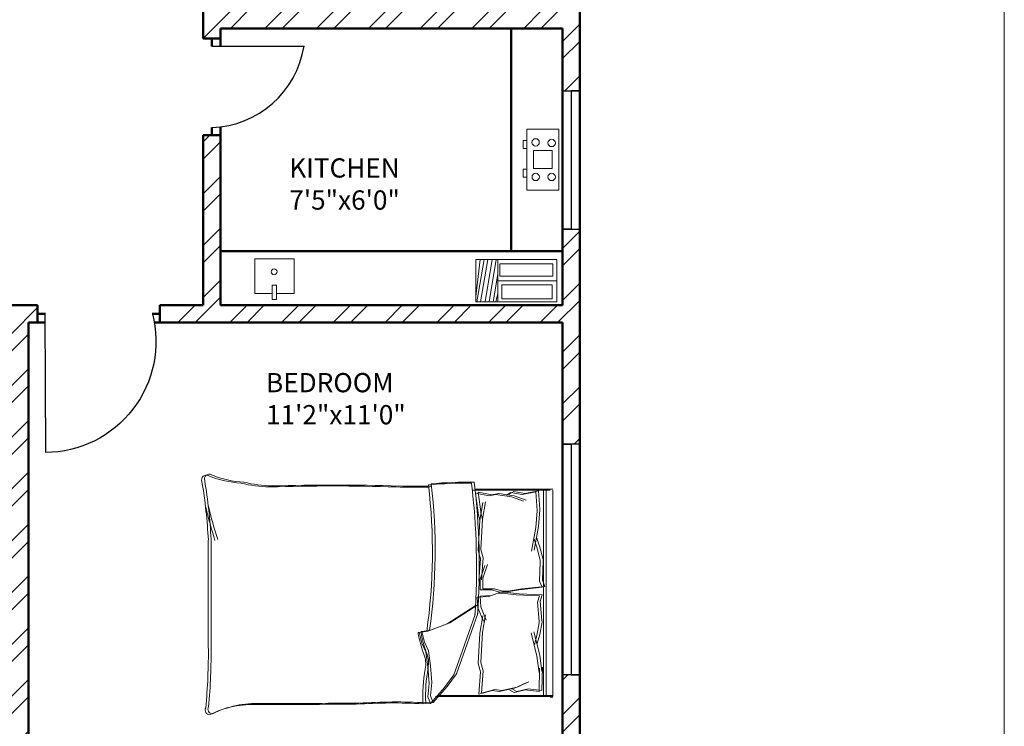
# Model space of a CAD drawing. Units: inches. Extents: x 1901 to 2863, y 888 to 2433.
# Tile 34 of 91: x 2607 to 2863, y 1291 to 1474. Entities that reach past the tile are written whole.
import ezdxf

# ---------------------------------------------------------------- set-up
doc = ezdxf.new("R2010")
doc.units = ezdxf.units.IN
for name, color, linetype, lineweight in [('A-AREA-IDEN', 7, 'Continuous', 18), ('A-DOOR', 4, 'Continuous', 25), ('A-FLOR-FIXT', 9, 'Continuous', 18), ('A-FURN', 8, 'Continuous', 18), ('A-GLAZ', 3, 'Continuous', 25), ('A-WALL', 7, 'Continuous', 50), ('A-WALL-PATT', 8, 'Continuous', 13)]:
    doc.layers.add(name, color=color, linetype=linetype, lineweight=lineweight)
doc.styles.get("Standard").update_dxf_attribs({"font": 'arial.ttf'})

# ---------------------------------------------------------------- blocks, each defined once
blk = doc.blocks.new('BED-DOUBLE')
for p, q in [((31.18, 59.32), (27.53, 55.16)), ((31.18, 59.32), (27.53, 55.16)), ((31.9, 59.58), (28.25, 55.42)), ((31.9, 59.58), (28.25, 55.42)), ((33.14, 59.41), (31.18, 59.32, 4.35)), ((33.14, 59.41), (31.18, 59.32, 4.35)), ((31.87, 57.59), (31.18, 59.32)), ((31.87, 57.59), (31.18, 59.32)), ((33.85, 59.67), (31.9, 59.58, 4.35)), ((33.85, 59.67), (31.9, 59.58, 4.35)), ((32.59, 57.85), (31.9, 59.58)), ((32.59, 57.85), (31.9, 59.58)), ((0.03, 57.78), (0.03, 4.12)), ((0.74, 57.78), (30.62, 57.78)), ((0.74, 57.78), (30.62, 57.78)), ((3.61, 56.48), (3.51, 50.42)), ((3.61, 56.48), (3.51, 50.42)), ((3.61, 56.48), (7.22, 56.06)), ((3.61, 56.48), (7.22, 56.06)), ((6.5, 55.8), (9.39, 56.47)), ((6.5, 55.8), (9.39, 56.47)), ((7.22, 56.06), (10.11, 56.73)), ((7.22, 56.06), (10.11, 56.73)), ((9.39, 56.47), (10.56, 55.89)), ((9.39, 56.47), (10.56, 55.89)), ((14.02, 56.48), (10.01, 55.58)), ((14.02, 56.48), (10.01, 55.58)), ((10.11, 56.73), (11.28, 56.15)), ((10.11, 56.73), (11.28, 56.15)), ((15.83, 56.27), (14.02, 56.48)), ((15.83, 56.27), (14.02, 56.48)), ((18.63, 56.89), (15.11, 56.01)), ((18.63, 56.88), (15.11, 56.01)), ((19.35, 57.14), (15.83, 56.27)), ((19.35, 57.14), (15.83, 56.27)), ((18.18, 51.12), (18.63, 56.89)), ((18.18, 51.12), (18.63, 56.88)), ((18.9, 51.38), (19.35, 57.14)), ((18.9, 51.38), (19.35, 57.14)), ((31.53, 54.12), (31.87, 57.59)), ((31.53, 54.12), (31.87, 57.59)), ((32.24, 54.37), (32.59, 57.85)), ((32.24, 54.37), (32.59, 57.85)), ((2.9, 56.23), (2.79, 50.16)), ((2.9, 56.23), (2.79, 50.16)), ((2.9, 56.23), (6.5, 55.8)), ((2.9, 56.23), (6.5, 55.8)), ((9.3, 55.33), (6.29, 54)), ((9.3, 55.33), (6.29, 54)), ((10.01, 55.58), (7.01, 54.26)), ((10.01, 55.58), (7.01, 54.26)), ((13.31, 56.23), (9.3, 55.33)), ((13.31, 56.23), (9.3, 55.33)), ((15.11, 56.01), (13.31, 56.23)), ((15.11, 56.01), (13.31, 56.23)), ((27.53, 55.16), (25.1, 51.86)), ((27.53, 55.16), (25.1, 51.86)), ((28.25, 55.42), (25.81, 52.11)), ((28.25, 55.42), (25.81, 52.11)), ((31.87, 49.77), (31.53, 54.12)), ((31.87, 49.77), (31.53, 54.12)), ((32.59, 50.03), (32.24, 54.37)), ((32.59, 50.03), (32.24, 54.37)), ((2.79, 50.16), (2.88, 51.29)), ((2.79, 50.16), (2.88, 51.29)), ((2.88, 51.29), (3.47, 47.02)), ((2.88, 51.29), (3.47, 47.02)), ((3.51, 50.42), (3.6, 51.54)), ((3.51, 50.42), (3.6, 51.54)), ((3.6, 51.54), (4.19, 47.28)), ((3.6, 51.54), (4.19, 47.28)), ((19.52, 49.18), (18.9, 51.38)), ((19.52, 49.18), (18.9, 51.38)), ((25.1, 51.86), (22.84, 45.6)), ((25.1, 51.86), (22.84, 45.6)), ((25.81, 52.11), (23.55, 45.85)), ((25.81, 52.11), (23.55, 45.85)), ((18.81, 48.92), (18.18, 51.12)), ((18.81, 48.92), (18.18, 51.12)), ((18.32, 41.05), (18.81, 48.92)), ((18.32, 41.05), (18.81, 48.92)), ((19.04, 41.31), (19.52, 49.18)), ((19.04, 41.31), (19.52, 49.18)), ((32.39, 45.94), (31.87, 49.77)), ((32.39, 45.94), (31.87, 49.77)), ((33.11, 46.2), (32.59, 50.03)), ((33.11, 46.2), (32.59, 50.03)), ((3.47, 47.02), (4.99, 40.94)), ((3.47, 47.02), (4.99, 40.94)), ((4.19, 47.28), (5.71, 41.19)), ((4.19, 47.28), (5.71, 41.19)), ((34.15, 43.94), (33.11, 46.2)), ((34.15, 43.94), (33.11, 46.2)), ((4.15, 43.98), (3.48, 41.66)), ((4.15, 43.98), (3.48, 41.66)), ((4.87, 44.23), (4.2, 41.91)), ((4.87, 44.23), (4.2, 41.91)), ((22.84, 45.6), (19.54, 36.24)), ((22.84, 45.6), (19.54, 36.24)), ((23.55, 45.85), (20.26, 36.49)), ((23.55, 45.85), (20.26, 36.49)), ((33.44, 43.68), (32.39, 45.94)), ((33.44, 43.68), (32.39, 45.94)), ((34.13, 40.9), (33.44, 43.68)), ((34.13, 40.9), (33.44, 43.68)), ((34.85, 41.16), (34.15, 43.94)), ((34.85, 41.16), (34.15, 43.94)), ((89, 16.88), (89, 44.51)), ((89, 16.88), (89, 44.51)), ((89.72, 17.13), (89.72, 44.77)), ((89.72, 17.13), (89.72, 44.77)), ((3.48, 41.66), (2.87, 38.37)), ((3.48, 41.66), (2.87, 38.37)), ((4.2, 41.91), (3.59, 38.62)), ((4.2, 41.91), (3.59, 38.62)), ((17.57, 36.53), (18.32, 41.05)), ((17.57, 36.52), (18.32, 41.05)), ((18.29, 36.78), (19.04, 41.31)), ((18.29, 36.78), (19.04, 41.31)), ((32.59, 40.81), (34.85, 41.16)), ((32.59, 40.81), (34.85, 41.16)), ((3.59, 38.62), (3.62, 38.26)), ((3.59, 38.62), (3.62, 38.26)), ((19.54, 33.94), (26.83, 38.64)), ((19.54, 33.94), (26.83, 38.64)), ((20.26, 34.19), (27.55, 38.9)), ((20.26, 34.19), (27.55, 38.9)), ((26.83, 38.64), (31.87, 40.55)), ((26.83, 38.64), (31.87, 40.55)), ((27.55, 38.9), (32.59, 40.81)), ((27.55, 38.9), (32.59, 40.81)), ((31.87, 40.55), (34.13, 40.9)), ((31.87, 40.55), (34.13, 40.9)), ((2.87, 38.37), (2.9, 38.01)), ((2.87, 38.37), (2.9, 38.01)), ((2.9, 38.01), (3.37, 33.03)), ((2.9, 38.01), (3.37, 33.04)), ((3.62, 38.26), (4.09, 33.29)), ((3.62, 38.26), (4.09, 33.29)), ((18.82, 34.49), (17.38, 37.94)), ((18.82, 34.49), (17.38, 37.94)), ((19.54, 34.74), (18.1, 38.19)), ((19.54, 34.74), (18.1, 38.19)), ((18.99, 31.73), (18.82, 34.49)), ((18.99, 31.73), (18.82, 34.49)), ((19.71, 31.99), (19.54, 34.74)), ((19.71, 31.99), (19.54, 34.74)), ((3.37, 33.04), (2.82, 31.37)), ((3.37, 33.03), (2.82, 31.37)), ((2.82, 31.37), (8.86, 31.1)), ((2.82, 31.37), (8.86, 31.1)), ((4.09, 33.29), (3.54, 31.63)), ((4.09, 33.29), (3.54, 31.63)), ((3.54, 31.63), (9.58, 31.36)), ((3.54, 31.63), (9.58, 31.36)), ((8.86, 31.1), (12.46, 30.68)), ((8.86, 31.1), (12.46, 30.68)), ((9.58, 31.36), (13.18, 30.93)), ((9.58, 31.36), (13.18, 30.93)), ((12.46, 30.68), (13.92, 30.77)), ((12.46, 30.68), (13.92, 30.77)), ((13.18, 30.93), (14.64, 31.02)), ((13.18, 30.93), (14.64, 31.02)), ((13.92, 30.77), (15.99, 31.55)), ((13.92, 30.77), (15.99, 31.55)), ((14.64, 31.02), (16.71, 31.8)), ((14.64, 31.02), (16.71, 31.8)), ((15.99, 31.55), (18.99, 31.73)), ((15.99, 31.55), (18.99, 31.73)), ((16.71, 31.8), (19.71, 31.99)), ((16.71, 31.8), (19.71, 31.99)), ((2.13, 29.14), (8.13, 29.78)), ((2.13, 29.14), (8.13, 29.78)), ((2.78, 27.51), (2.13, 29.14)), ((2.78, 27.51), (2.13, 29.14)), ((2.84, 29.39), (8.85, 30.04)), ((2.84, 29.39), (8.85, 30.04)), ((3.49, 27.77), (2.84, 29.39)), ((3.49, 27.77), (2.84, 29.39)), ((8.13, 29.78), (11.7, 30.43)), ((8.13, 29.78), (11.7, 30.43)), ((8.85, 30.04), (12.42, 30.69)), ((8.85, 30.04), (12.42, 30.69)), ((11.7, 30.43), (13.16, 30.43)), ((11.7, 30.43), (13.16, 30.43)), ((12.42, 30.69), (13.88, 30.69)), ((12.42, 30.69), (13.88, 30.69)), ((13.16, 30.43), (15.28, 29.78)), ((13.16, 30.43), (15.28, 29.78)), ((13.88, 30.69), (15.99, 30.04)), ((13.88, 30.69), (15.99, 30.04)), ((15.28, 29.78), (18.29, 29.78)), ((15.28, 29.78), (18.29, 29.78)), ((15.99, 30.04), (19, 30.04)), ((15.99, 30.04), (19, 30.04)), ((18.29, 29.78), (18.29, 27.03)), ((18.29, 29.78), (18.29, 27.03)), ((19, 30.04), (19, 27.28)), ((19, 30.04), (19, 27.28)), ((2.61, 22.52), (2.78, 27.51)), ((2.61, 22.52), (2.78, 27.51)), ((3.33, 22.78), (3.49, 27.77)), ((3.33, 22.78), (3.49, 27.77)), ((18.29, 27.03), (17.06, 23.49)), ((18.29, 27.03), (17.06, 23.5)), ((19, 27.28), (17.78, 23.75)), ((19, 27.28), (17.78, 23.75)), ((18.18, 21.73), (18.63, 27.49)), ((18.18, 21.73), (18.63, 27.49)), ((18.9, 21.98), (19.35, 27.75)), ((18.9, 21.98), (19.35, 27.74)), ((2.61, 22.16), (2.61, 22.52)), ((2.61, 22.16), (2.61, 22.52)), ((3.42, 18.91), (2.61, 22.16)), ((3.42, 18.91), (2.61, 22.16)), ((3.33, 22.42), (3.33, 22.78)), ((3.33, 22.42), (3.33, 22.78)), ((4.14, 19.17), (3.33, 22.42)), ((4.14, 19.17), (3.33, 22.42)), ((18.81, 19.53), (18.18, 21.73)), ((18.81, 19.53), (18.18, 21.73)), ((19.52, 19.78), (18.9, 21.98)), ((19.52, 19.78), (18.9, 21.98)), ((4.24, 16.64), (3.42, 18.91)), ((4.24, 16.64), (3.42, 18.91)), ((3.75, 13.56), (4.89, 19.73)), ((3.75, 13.56), (4.89, 19.73)), ((4.95, 16.9), (4.14, 19.17)), ((4.95, 16.9), (4.14, 19.17)), ((4.47, 13.81), (5.6, 19.98)), ((4.47, 13.81), (5.6, 19.98)), ((18.32, 11.66), (18.81, 19.53)), ((18.32, 11.66), (18.81, 19.53)), ((19.04, 11.91), (19.52, 19.78)), ((19.04, 11.91), (19.52, 19.78)), ((3.42, 9.27), (3.75, 13.56)), ((3.42, 9.27), (3.75, 13.56)), ((4.14, 9.52), (4.47, 13.81)), ((4.14, 9.52), (4.47, 13.81)), ((17.57, 7.13), (18.32, 11.66)), ((17.57, 7.13), (18.32, 11.66)), ((18.29, 7.38), (19.04, 11.91)), ((18.29, 7.39), (19.04, 11.91)), ((18.32, 11.66), (18.68, 10.38)), ((18.32, 11.66), (18.68, 10.38)), ((18.68, 10.38), (19.5, 4.66)), ((18.68, 10.38), (19.5, 4.66)), ((19.04, 11.91), (19.4, 10.64)), ((19.04, 11.91), (19.4, 10.64)), ((19.4, 10.64), (20.21, 4.92)), ((19.4, 10.64), (20.21, 4.92)), ((3.4, 9.15), (3.42, 9.27)), ((3.4, 9.15), (3.42, 9.27)), ((3.77, 4.34), (3.4, 9.15)), ((3.77, 4.34), (3.4, 9.15)), ((4.12, 9.4), (4.14, 9.52)), ((4.12, 9.4), (4.14, 9.52)), ((4.49, 4.6), (4.12, 9.4)), ((4.49, 4.6), (4.12, 9.4)), ((4.47, 4.59), (8.04, 5.24)), ((4.47, 4.59), (8.04, 5.24)), ((10.08, 5.63), (7, 6.77)), ((10.08, 5.63), (7, 6.77)), ((10.8, 5.89), (7.71, 7.03)), ((10.8, 5.89), (7.71, 7.03)), ((8.04, 5.24), (10.96, 4.75)), ((8.04, 5.24), (10.96, 4.76)), ((14.14, 4.99), (10.08, 5.63)), ((14.14, 4.99), (10.08, 5.63)), ((10.24, 4.5), (11.38, 5.15)), ((10.24, 4.5), (11.38, 5.15)), ((14.86, 5.24), (10.8, 5.89)), ((14.86, 5.24), (10.8, 5.89)), ((10.96, 4.76), (12.1, 5.4)), ((10.96, 4.75), (12.1, 5.4)), ((15.92, 5.31), (14.14, 4.99)), ((15.92, 5.31), (14.14, 4.99)), ((16.64, 5.57), (14.86, 5.24)), ((16.64, 5.57), (14.86, 5.24)), ((19.5, 4.66), (15.92, 5.31)), ((19.5, 4.66), (15.92, 5.31)), ((20.21, 4.92), (16.64, 5.57)), ((20.21, 4.92), (16.64, 5.57)), ((3.75, 4.34), (7.32, 4.99)), ((3.75, 4.34), (7.32, 4.99)), ((7.32, 4.99), (10.24, 4.5)), ((7.32, 4.99), (10.24, 4.5))]:
    blk.add_line(p, q)
for centre, radius, start, end in [((77.12, 85.47), 25.9, 267.4714, 296.4681), ((77.12, 85.47), 25.9, 267.4714, 296.4681), ((77.84, 85.73), 25.9, 267.4714, 296.4681), ((77.84, 85.73), 25.9, 267.4714, 296.4681), ((88.58, 61.05), 1.24, 332.6588, 86.02), ((88.58, 61.05), 1.24, 332.6588, 86.02), ((89.3, 61.31), 1.24, 332.6588, 86.02), ((89.3, 61.31), 1.24, 332.6588, 86.02), ((-7.45, 57.59), 40.62, 349.8763, 2.5657), ((-7.45, 57.59), 40.62, 349.8763, 2.5657), ((40.8, 204.6), 145.39, 266.9791, 273.8365), ((40.8, 204.6), 145.39, 266.9791, 273.8365), ((-6.73, 57.85), 40.62, 349.8763, 2.5657), ((-6.73, 57.85), 40.62, 349.8763, 2.5657), ((41.52, 204.86), 145.39, 266.9791, 273.8365), ((41.52, 204.86), 145.39, 266.9791, 273.8365), ((76.17, -5062.23), 5121.82, 90.00217, 90.28689), ((76.17, -5062.23), 5121.82, 90.00217, 90.28689), ((76.89, -5061.97), 5121.82, 90.00217, 90.28689), ((76.89, -5061.97), 5121.82, 90.00217, 90.28689), ((238.36, 46.17), 149.37, 174.4998, 180.6351), ((238.36, 46.17), 149.37, 174.4998, 180.6351), ((239.08, 46.42), 149.37, 174.4998, 180.6351), ((239.08, 46.42), 149.37, 174.4998, 180.6351), ((39.4, 49.08), 6.99, 168.6608, 203.7384), ((39.4, 49.08), 6.99, 168.6608, 203.7384), ((40.11, 49.33), 6.99, 168.6608, 203.7384), ((40.11, 49.33), 6.99, 168.6608, 203.7384), ((1.69, 34.94), 33.29, 10.6617, 19.8806), ((1.69, 34.94), 33.29, 10.6617, 19.8806), ((2.41, 35.2), 33.29, 10.6617, 19.8806), ((2.41, 35.2), 33.29, 10.6617, 19.8806), ((34.2, 41.1), 0.207, 250.2464, 1.1377), ((34.2, 41.1), 0.207, 250.2464, 1.1377), ((34.92, 41.35), 0.207, 250.2464, 1.1377), ((34.92, 41.35), 0.207, 250.2464, 1.1377), ((175.53, 19.9), 144.86, 171.7845, 186.9006), ((175.53, 19.9), 144.86, 171.7845, 186.9006), ((176.25, 20.16), 144.86, 171.7845, 186.9006), ((176.25, 20.15), 144.86, 171.7845, 186.9006), ((204.43, 23.94), 185.22, 176.0865, 186.7821), ((204.43, 23.94), 185.22, 176.0865, 186.7821), ((205.14, 24.2), 185.22, 176.0865, 186.7821), ((205.14, 24.2), 185.22, 176.0865, 186.7821), ((225.52, 24.02), 136.7, 182.9958, 189.4091), ((225.52, 24.02), 136.7, 182.9958, 189.4091), ((226.23, 24.28), 136.7, 182.9958, 189.4091), ((226.23, 24.28), 136.7, 182.9958, 189.4091), ((23.31, 95.84), 93.53, 268.7218, 275.604), ((23.31, 95.84), 93.53, 268.7218, 275.604), ((35.03, -187.88), 190.99, 88.4762, 91.0082), ((35.03, -187.88), 190.99, 88.4762, 91.0082), ((35.74, -187.62), 190.99, 88.4762, 91.0082), ((35.74, -187.62), 190.99, 88.4762, 91.0082), ((56.85, 544.3), 541.51, 268.2277, 271.7185), ((56.85, 544.3), 541.51, 268.2277, 271.7185), ((57.57, 544.55), 541.51, 268.2277, 271.7185), ((57.57, 544.55), 541.51, 268.2277, 271.7185), ((72.46, -30.24), 33.27, 76.0648, 88.9113), ((72.46, -30.24), 33.27, 76.0648, 88.9113), ((73.18, -29.98), 33.27, 76.0648, 88.9113), ((73.18, -29.98), 33.27, 76.0648, 88.9113), ((22.59, 95.58), 93.53, 268.7218, 275.604), ((22.59, 95.58), 93.53, 268.7218, 275.604), ((78.93, -24.35), 26.45, 67.9751, 86.652), ((78.93, -24.35), 26.45, 67.9751, 86.652), ((79.65, -24.1), 26.45, 67.9751, 86.652), ((79.65, -24.1), 26.45, 67.9751, 86.652), ((89.53, 1.18), 1.22, 236.1736, 23.4781), ((89.53, 1.18), 1.22, 236.1736, 23.4781), ((90.25, 1.44), 1.22, 236.1736, 23.4781), ((90.25, 1.44), 1.22, 236.1736, 23.4781)]:
    blk.add_arc(centre, radius, start, end)
blk = doc.blocks.new('WIN-60')
for p, q in [((0, 4.5), (0, 0)), ((60, 2.25), (60, 4.5)), ((60, 4.5), (60, 0)), ((0, 0), (0, 2.25)), ((0, 2.25), (60, 2.25))]:
    blk.add_line(p, q)
blk = doc.blocks.new('WIN-36-5')
for p, q in [((0, 36), (4.5, 36)), ((4.5, 36), (2.25, 36)), ((2.25, 36), (2.25, 0)), ((2.25, 0), (0, 0)), ((0, 0), (4.5, 0))]:
    blk.add_line(p, q)
blk = doc.blocks.new('DOOR-29')
blk.add_line((0, -0.02), (0, 35.98))
blk.add_arc((0, 7.12), 28.86, 345.6888, 90)

msp = doc.modelspace()

# ---------------------------------------------------------------- hatches: boundary and pattern name
at = {"layer": 'A-WALL-PATT'}
h = msp.add_hatch(dxfattribs=at)
h.set_pattern_fill('ANSI32', color=256)
h.paths.add_polyline_path([(2192.5, 2274.13), (2141.26, 2274.13), (2141.26, 2269.63), (2192.5, 2269.63)])
h.paths.add_polyline_path([(2259.93, 2274.13), (2216.5, 2274.13), (2216.5, 2269.63), (2255.43, 2269.63), (2255.43, 2214.63), (2250.81, 2214.63), (2250.81, 2210.13), (2259.93, 2210.13), (2259.93, 2215.13), (2271.76, 2215.13), (2271.76, 2217.38), (2271.76, 2219.63), (2259.93, 2219.63)])
h.paths.add_polyline_path([(2171.43, 2269.63), (2166.93, 2269.63), (2166.93, 2219.63), (2121.24, 2219.63), (2121.24, 2215.13), (2166.93, 2215.13), (2166.93, 2083.13), (2161.81, 2083.13), (2161.81, 2078.63), (2171.43, 2078.63), (2177, 2078.63), (2177, 2080.88), (2177, 2083.13), (2171.43, 2083.13), (2171.43, 2210.13), (2230.91, 2210.13), (2230.91, 2212.38), (2230.91, 2214.63), (2171.43, 2214.63)])
h.paths.add_polyline_path([(2117.26, 2274.13), (2089.43, 2274.13), (2089.43, 2219.63), (2081.14, 2219.63), (2081.14, 2215.13), (2089.43, 2215.13), (2098, 2215.13), (2098, 2217.38), (2098, 2219.63), (2093.93, 2219.63), (2093.93, 2269.63), (2117.26, 2269.63), (2117.26, 2271.88)])
h.paths.add_polyline_path([(2343.43, 2219.63), (2329.29, 2219.63), (2329.29, 2215.13), (2338.93, 2215.13), (2338.93, 2184.74), (2343.43, 2184.74)])
h.paths.add_polyline_path([(2338.93, 2083.13), (2329.29, 2083.13), (2208.97, 2083.13), (2208.97, 2078.63), (2338.93, 2078.63)])
h.paths.add_polyline_path([(2343.43, 2136.74), (2338.93, 2136.74), (2338.93, 1872.63), (2343.43, 1872.63)])
h.paths.add_polyline_path([(2343.43, 1863.63), (2397.68, 1863.63), (2397.68, 1821.63), (2384.14, 1821.63), (2384.14, 1812.63), (2418.33, 1812.63), (2418.33, 1817.13), (2418.33, 1821.63), (2406.68, 1821.63), (2406.68, 1863.63), (2459.5, 1863.63), (2459.5, 1821.63), (2447.14, 1821.63), (2447.14, 1812.63), (2459.5, 1812.63), (2468.5, 1812.63), (2468.5, 1872.63), (2394.43, 1872.63), (2334.43, 1872.63), (2334.43, 1812.63), (2343.43, 1812.63), (2353.25, 1812.63), (2353.25, 1821.63), (2343.43, 1821.63)])
h.paths.add_polyline_path([(2510.01, 1872.63), (2468.5, 1872.63), (2468.5, 1868.13), (2510.01, 1868.13)])
h.paths.add_polyline_path([(2514.01, 1817.13), (2468.5, 1817.13), (2468.5, 1812.63), (2482.11, 1812.63), (2482.11, 1800.61), (2486.61, 1800.61), (2486.61, 1812.63), (2514.01, 1812.63)])
h.paths.add_polyline_path([(2299.25, 1814.88), (2299.25, 1817.13), (2295.93, 1817.13), (2295.93, 1854.17), (2293.68, 1854.17), (2291.43, 1854.17), (2291.43, 1817.13), (2266.11, 1817.13), (2266.11, 1812.63), (2299.25, 1812.63)])
h.paths.add_polyline_path([(2218.11, 1817.13), (2206.46, 1817.13), (2171.43, 1817.13), (2171.43, 1949.13), (2190.1, 1949.13), (2190.1, 1953.63), (2163.47, 1953.63), (2163.47, 1949.13), (2166.93, 1949.13), (2166.93, 1817.13), (2114.3, 1817.13), (2114.3, 1812.63), (2218.11, 1812.63)])
h.paths.add_polyline_path([(2029.43, 1970.92), (2024.93, 1970.92), (2024.93, 1912.72), (2029.43, 1912.72)])
h.paths.add_polyline_path([(2132.3, 1953.63), (2113.93, 1953.63), (2113.93, 1975.89), (2111.68, 1975.89), (2109.43, 1975.89), (2109.43, 1953.63), (2029.43, 1953.63), (2029.43, 1949.13), (2132.3, 1949.13)])
h.paths.add_polyline_path([(2029.43, 1853.61), (2029.31, 1853.61), (2029.31, 1853.61), (2029.43, 1853.61), (2029.43, 1864.72), (2024.93, 1864.72), (2024.93, 1812.63), (2066.3, 1812.63), (2066.3, 1814.88), (2066.3, 1817.13), (2029.43, 1817.13)])
h.paths.add_polyline_path([(2122.93, 2010.09), (2120.68, 2010.09), (2118.43, 2010.09), (2118.43, 2006.13), (2029.43, 2006.13), (2029.43, 2001.63), (2109.43, 2001.63), (2109.43, 1998.04), (2113.93, 1998.04), (2113.93, 2001.63), (2122.93, 2001.63)])
h.paths.add_polyline_path([(2029.43, 2031.38), (2024.93, 2031.38), (2024.93, 1994.92), (2027.18, 1994.92), (2029.43, 1994.92)])
h.paths.add_polyline_path([(2029.43, 2136.74), (2024.93, 2136.74), (2024.93, 2067.38), (2027.18, 2067.38), (2029.43, 2067.38)])
h.paths.add_polyline_path([(2125.62, 2083.13), (2029.43, 2083.13), (2029.43, 2078.63), (2118.43, 2078.63), (2118.43, 2030.71), (2122.93, 2030.71), (2122.93, 2078.63), (2125.62, 2078.63)])
h.paths.add_polyline_path([(2029.43, 2215.13), (2040.47, 2215.13), (2040.47, 2217.38), (2040.47, 2219.63), (2024.93, 2219.63), (2024.93, 2184.74), (2029.43, 2184.74), (2029.43, 2187.78)])
h.paths.add_polyline_path([(2686.43, 2274.13), (2659.28, 2274.13), (2659.28, 2269.63), (2681.93, 2269.63), (2681.93, 2219.63), (2676.82, 2219.63), (2676.82, 2215.13), (2681.93, 2215.13), (2697.01, 2215.13), (2697.01, 2217.38), (2697.01, 2219.63), (2686.43, 2219.63)])
h.paths.add_polyline_path([(2609.93, 2269.63), (2635.28, 2269.63), (2635.28, 2274.13), (2571.43, 2274.13), (2571.43, 2269.63), (2605.43, 2269.63), (2605.43, 2214.63), (2549.1, 2214.63), (2549.1, 2210.13), (2605.43, 2210.13), (2605.43, 2083.13), (2601.01, 2083.13), (2601.01, 2080.88), (2601.01, 2078.63), (2609.93, 2078.63), (2616.16, 2078.63), (2616.16, 2080.88), (2616.16, 2083.13), (2609.93, 2083.13), (2609.93, 2215.13), (2651.46, 2215.13), (2651.46, 2217.38), (2651.46, 2219.63), (2609.93, 2219.63)])
h.paths.add_polyline_path([(2521.43, 2269.63), (2547.43, 2269.63), (2547.43, 2271.88), (2547.43, 2274.13), (2516.93, 2274.13), (2516.93, 2219.63), (2506.41, 2219.63), (2506.41, 2215.13), (2516.93, 2215.13), (2516.93, 2210.13), (2525.4, 2210.13), (2525.4, 2212.38), (2525.4, 2214.63), (2521.43, 2214.63)])
h.paths.add_polyline_path([(2456.01, 2219.63), (2439.43, 2219.63), (2439.43, 2187.89), (2443.93, 2187.89), (2443.93, 2215.13), (2456.01, 2215.13)])
h.paths.add_polyline_path([(2752.93, 2219.63), (2739.48, 2219.63), (2739.48, 2215.13), (2748.43, 2215.13), (2748.43, 2187.89), (2752.93, 2187.89)])
h.paths.add_polyline_path([(2752.93, 2139.89), (2748.43, 2139.89), (2748.43, 2083.13), (2648.42, 2083.13), (2648.42, 2078.63), (2654.93, 2078.63), (2654.93, 2039.44), (2659.43, 2039.44), (2659.43, 2078.63), (2748.43, 2078.63), (2748.43, 2063.43), (2752.93, 2063.43)])
h.paths.add_polyline_path([(2752.93, 2010.63), (2659.43, 2010.63), (2659.43, 2015.65), (2654.93, 2015.65), (2654.93, 2010.63), (2605.43, 2010.63), (2605.43, 1920.97), (2609.93, 1920.97), (2609.93, 2006.13), (2748.43, 2006.13), (2748.43, 1982.47), (2752.93, 1982.47)])
h.paths.add_polyline_path([(2752.93, 2027.43), (2748.43, 2027.43), (2748.43, 2010.63), (2752.93, 2010.63)])
h.paths.add_polyline_path([(2748.43, 1886.13), (2609.93, 1886.13), (2609.93, 1889.72), (2605.43, 1889.72), (2605.43, 1861.26), (2609.93, 1861.26), (2609.93, 1881.63), (2748.43, 1881.63)])
h.paths.add_polyline_path([(2456.86, 2228.83), (2498.4, 2228.83), (2498.4, 2247.49), (2456.86, 2247.49)], flags=9)
h.paths.add_polyline_path([(2038.6, 2237.42), (2080.17, 2237.42), (2080.17, 2256.08), (2038.6, 2256.08)], flags=9)
h.paths.add_polyline_path([(2292.01, 1062.39), (2539.93, 1062.39), (2539.93, 1099.49), (2292.01, 1099.49)], flags=9)
h.paths.add_polyline_path([(2424.91, 1832.25), (2448.51, 1832.25), (2448.51, 1846.68), (2424.91, 1846.68)], flags=25)
h.paths.add_polyline_path([(2359.08, 1832.25), (2382.68, 1832.25), (2382.68, 1846.68), (2359.08, 1846.68)], flags=25)
h.paths.add_polyline_path([(2352.9, 1684.8), (2367.54, 1684.8), (2367.54, 1697.17), (2352.9, 1697.17)], flags=9)
h.paths.add_polyline_path([(2079.29, 1755.83), (2169.02, 1755.83), (2169.02, 1774.37), (2079.29, 1774.37)], flags=9)
h.paths.add_polyline_path([(2404.09, 1373.86), (2404.09, 1463.59), (2385.54, 1463.59), (2385.54, 1373.86)], flags=9)
h.paths.add_polyline_path([(2268.09, 2236.37), (2309.64, 2236.37), (2309.64, 2255.03), (2268.09, 2255.03)], flags=9)
h.paths.add_polyline_path([(2575.96, 1700.95), (2665.7, 1700.95), (2665.7, 1719.5), (2575.96, 1719.5)], flags=9)
h.paths.add_polyline_path([(2302.96, 1878.47), (2329.52, 1878.47), (2329.52, 1888.78), (2302.96, 1888.78)], flags=9)
h.paths.add_polyline_path([(2097.42, 2240.58), (2126.57, 2240.58), (2126.57, 2259.23), (2097.42, 2259.23)], flags=9)
h.paths.add_polyline_path([(2208.72, 2246.12), (2237.88, 2246.12), (2237.88, 2264.78), (2208.72, 2264.78)], flags=9)
h.paths.add_polyline_path([(2038.15, 1925.96), (2076.99, 1925.96), (2076.99, 1944.62), (2038.15, 1944.62)], flags=9)
h.paths.add_polyline_path([(2239.14, 1926.67), (2288.46, 1926.67), (2288.46, 1945.33), (2239.14, 1945.33)], flags=9)
h.paths.add_polyline_path([(2175.43, 2007.33), (2212.36, 2007.33), (2212.36, 2025.99), (2175.43, 2025.99)], flags=9)
h.paths.add_polyline_path([(2225.03, 2091.79), (2263.87, 2091.79), (2263.87, 2110.45), (2225.03, 2110.45)], flags=9)
h.paths.add_polyline_path([(2035.4, 2098.48), (2074.24, 2098.48), (2074.24, 2117.14), (2035.4, 2117.14)], flags=9)
h.paths.add_polyline_path([(2050.1, 2029.21), (2083.26, 2029.21), (2083.26, 2047.87), (2050.1, 2047.87)], flags=9)
h.paths.add_polyline_path([(2069.68, 1956.72), (2098.83, 1956.72), (2098.83, 1975.38), (2069.68, 1975.38)], flags=25)
h.paths.add_polyline_path([(2328.62, 1753.34), (2361.66, 1753.34), (2361.66, 1771.99), (2328.62, 1771.99)], flags=9)
h.paths.add_polyline_path([(2395.16, 2060.89), (2395.16, 2140.65), (2378.68, 2140.65), (2378.68, 2060.89)], flags=9)
h.paths.add_polyline_path([(2463.73, 2059.02), (2492.89, 2059.02), (2492.89, 2077.68), (2463.73, 2077.68)], flags=9)
h.paths.add_polyline_path([(2458.03, 2181.54), (2496.87, 2181.54), (2496.87, 2200.19), (2458.03, 2200.19)], flags=9)
h.paths.add_polyline_path([(2527.58, 2243.07), (2556.73, 2243.07), (2556.73, 2261.73), (2527.58, 2261.73)], flags=9)
h.paths.add_polyline_path([(2694.46, 2232.77), (2736.03, 2232.77), (2736.03, 2251.42), (2694.46, 2251.42)], flags=9)
h.paths.add_polyline_path([(2637.82, 2249.22), (2666.98, 2249.22), (2666.98, 2267.88), (2637.82, 2267.88)], flags=9)
h.paths.add_polyline_path([(2623.69, 2183.54), (2662.53, 2183.54), (2662.53, 2202.2), (2623.69, 2202.2)], flags=9)
h.paths.add_polyline_path([(2691.97, 2021.5), (2725.12, 2021.5), (2725.12, 2040.16), (2691.97, 2040.16)], flags=9)
h.paths.add_polyline_path([(2621.04, 1975.91), (2662.34, 1975.91), (2662.34, 1994.57), (2621.04, 1994.57)], flags=25)
h.paths.add_polyline_path([(2479.03, 1927.62), (2519.84, 1927.62), (2519.84, 1946.28), (2479.03, 1946.28)], flags=9)
h.paths.add_polyline_path([(2670.94, 1849.08), (2716.01, 1849.08), (2716.01, 1867.73), (2670.94, 1867.73)], flags=9)
h.paths.add_polyline_path([(2523.61, 1782.96), (2550.17, 1782.96), (2550.17, 1793.26), (2523.61, 1793.26)], flags=9)
h.paths.add_polyline_path([(2450.84, 1207.33), (2492.39, 1207.33), (2492.39, 1225.99), (2450.84, 1225.99)], flags=9)
h.paths.add_polyline_path([(2527.75, 1203.84), (2556.91, 1203.84), (2556.91, 1222.5), (2527.75, 1222.5)], flags=9)
h.paths.add_polyline_path([(2639.11, 1207.2), (2668.27, 1207.2), (2668.27, 1225.86), (2639.11, 1225.86)], flags=9)
h.paths.add_polyline_path([(2692.59, 1218.97), (2734.17, 1218.97), (2734.17, 1237.62), (2692.59, 1237.62)], flags=9)
h.paths.add_polyline_path([(2669.27, 1366.33), (2708.11, 1366.33), (2708.11, 1384.99), (2669.27, 1384.99)], flags=9)
h.paths.add_polyline_path([(2463.31, 1358.03), (2502.15, 1358.03), (2502.15, 1376.69), (2463.31, 1376.69)], flags=9)
h.paths.add_polyline_path([(2494.72, 1449.96), (2531.65, 1449.96), (2531.65, 1468.62), (2494.72, 1468.62)], flags=9)
h.paths.add_polyline_path([(2675.57, 1422.16), (2708.72, 1422.16), (2708.72, 1440.81), (2675.57, 1440.81)], flags=9)
h.paths.add_polyline_path([(2685.63, 1493.89), (2714.79, 1493.89), (2714.79, 1512.55), (2685.63, 1512.55)], flags=9)
h.paths.add_polyline_path([(2686.8, 1529.91), (2725.65, 1529.91), (2725.65, 1548.57), (2686.8, 1548.57)], flags=9)
h.paths.add_polyline_path([(2503.65, 1537.99), (2552.97, 1537.99), (2552.97, 1556.65), (2503.65, 1556.65)], flags=9)
h.paths.add_polyline_path([(2291.71, 1643.5), (2318.28, 1643.5), (2318.28, 1653.81), (2291.71, 1653.81)], flags=9)
h.paths.add_polyline_path([(2450.63, 1610.52), (2477.19, 1610.52), (2477.19, 1620.82), (2450.63, 1620.82)], flags=9)
h.paths.add_polyline_path([(2359.99, 1551.81), (2422.25, 1551.81), (2422.25, 1562.12), (2359.99, 1562.12)], flags=9)
h.paths.add_polyline_path([(2280.11, 1249.01), (2321.65, 1249.01), (2321.65, 1267.66), (2280.11, 1267.66)], flags=9)
h.paths.add_polyline_path([(2164.06, 1274.23), (2193.22, 1274.23), (2193.22, 1292.89), (2164.06, 1292.89)], flags=9)
h.paths.add_polyline_path([(2118.21, 1277.69), (2151.25, 1277.69), (2151.25, 1296.35), (2118.21, 1296.35)], flags=9)
h.paths.add_polyline_path([(2031.95, 1268.53), (2073.52, 1268.53), (2073.52, 1287.19), (2031.95, 1287.19)], flags=9)
h.paths.add_polyline_path([(2050.2, 1409.08), (2089.04, 1409.08), (2089.04, 1427.74), (2050.2, 1427.74)], flags=9)
h.paths.add_polyline_path([(2243.74, 1421.03), (2282.58, 1421.03), (2282.58, 1439.69), (2243.74, 1439.69)], flags=9)
h.paths.add_polyline_path([(2190.75, 1509.77), (2231.56, 1509.77), (2231.56, 1528.43), (2190.75, 1528.43)], flags=9)
h.paths.add_polyline_path([(2058.39, 1475.42), (2091.55, 1475.42), (2091.55, 1494.07), (2058.39, 1494.07)], flags=9)
h.paths.add_polyline_path([(2062.45, 1553.09), (2091.6, 1553.09), (2091.6, 1571.75), (2062.45, 1571.75)], flags=9)
h.paths.add_polyline_path([(2219.52, 1590.37), (2266.15, 1590.37), (2266.15, 1609.02), (2219.52, 1609.02)], flags=9)
h.paths.add_polyline_path([(2041.07, 1584.19), (2079.91, 1584.19), (2079.91, 1602.85), (2041.07, 1602.85)], flags=9)
h = msp.add_hatch(dxfattribs=at)
h.set_pattern_fill('ANSI32', color=256)
h.paths.add_polyline_path([(2443.93, 2139.89), (2439.43, 2139.89), (2439.43, 2069.35), (2441.68, 2069.35), (2443.93, 2069.35), (2443.93, 2078.63), (2521.93, 2078.63), (2521.93, 2075.07), (2524.18, 2075.07), (2526.43, 2075.07), (2526.43, 2078.63), (2571.75, 2078.63), (2571.75, 2080.88), (2571.75, 2083.13), (2443.93, 2083.13)])
h.paths.add_polyline_path([(2526.43, 2054.63), (2524.18, 2054.63), (2521.93, 2054.63), (2521.93, 2030.63), (2443.93, 2030.63), (2443.93, 2045.35), (2439.43, 2045.35), (2439.43, 1983.87), (2443.93, 1983.87), (2443.93, 2026.13), (2521.93, 2026.13), (2526.43, 2026.13)])
h.paths.add_polyline_path([(2443.93, 1923.87), (2439.43, 1923.87), (2439.43, 1872.63), (2443.93, 1872.63)])
h.paths.add_polyline_path([(2636.23, 1766.13), (2609.93, 1766.13), (2609.93, 1779.79), (2605.43, 1779.79), (2605.43, 1766.13), (2486.61, 1766.13), (2486.61, 1770.67), (2482.11, 1770.67), (2482.11, 1766.13), (2482.11, 1761.63), (2636.23, 1761.63), (2636.23, 1763.88)])
h.paths.add_polyline_path([(2519.54, 1663.38), (2519.54, 1665.63), (2494.93, 1665.63), (2481.83, 1665.63), (2481.83, 1663.38), (2481.83, 1661.13), (2490.43, 1661.13), (2490.43, 1640.16), (2494.93, 1640.16), (2494.93, 1661.13), (2519.54, 1661.13)])
h.paths.add_polyline_path([(2443.93, 1712.13), (2443.93, 1716.63), (2414.46, 1716.63), (2414.46, 1712.13), (2439.43, 1712.13), (2439.43, 1545.51), (2443.93, 1545.51), (2443.93, 1661.13), (2448.47, 1661.13), (2448.47, 1665.63), (2443.93, 1665.63)])
h.paths.add_polyline_path([(2343.43, 1712.13), (2365.52, 1712.13), (2365.52, 1714.38), (2365.52, 1716.63), (2333.87, 1716.63), (2333.87, 1714.38), (2333.87, 1712.13), (2338.93, 1712.13), (2338.93, 1575.63), (2338.93, 1545.51), (2343.43, 1545.51), (2343.43, 1547.51), (2343.43, 1580.13)])
h.paths.add_polyline_path([(2752.93, 1665.63), (2579.54, 1665.63), (2579.54, 1661.13), (2615.93, 1661.13), (2615.93, 1529.13), (2598.93, 1529.13), (2598.93, 1524.63), (2623.13, 1524.63), (2623.13, 1526.88), (2623.13, 1529.13), (2620.43, 1529.13), (2620.43, 1661.13), (2748.43, 1661.13), (2748.43, 1633.5), (2752.93, 1633.5)])
h.paths.add_polyline_path([(2752.93, 1419.93), (2748.43, 1419.93), (2748.43, 1400.13), (2659.43, 1400.13), (2659.43, 1444.33), (2657.18, 1444.33), (2654.93, 1444.33), (2654.93, 1400.13), (2643.65, 1400.13), (2643.65, 1395.63), (2748.43, 1395.63), (2748.43, 1364.04), (2752.93, 1364.04)])
h.paths.add_polyline_path([(2752.93, 1492.88), (2748.43, 1492.88), (2748.43, 1476.63), (2667.43, 1476.63), (2667.43, 1479.71), (2665.18, 1479.71), (2662.93, 1479.71), (2662.93, 1476.63), (2654.93, 1476.63), (2654.93, 1469.54), (2659.43, 1469.54), (2659.43, 1472.13), (2748.43, 1472.13), (2748.43, 1455.93), (2752.93, 1455.93)])
h.paths.add_polyline_path([(2752.93, 1304.04), (2748.43, 1304.04), (2748.43, 1263.63), (2738.66, 1263.63), (2738.66, 1259.13), (2752.93, 1259.13)])
h.paths.add_polyline_path([(2685.93, 1259.13), (2695.49, 1259.13), (2695.49, 1261.38), (2695.49, 1263.63), (2677.84, 1263.63), (2677.84, 1261.38), (2677.84, 1259.13), (2681.43, 1259.13), (2681.43, 1203.63), (2653.28, 1203.63), (2653.28, 1199.13), (2685.93, 1199.13), (2685.93, 1203.63)])
h.paths.add_polyline_path([(2609.43, 1395.63), (2611.85, 1395.63), (2611.85, 1400.13), (2598.89, 1400.13), (2598.89, 1397.88), (2598.89, 1395.63), (2604.93, 1395.63), (2604.93, 1268.13), (2554.73, 1268.13), (2554.73, 1265.88), (2554.73, 1263.63), (2604.93, 1263.63), (2604.93, 1203.63), (2571.31, 1203.63), (2571.31, 1199.13), (2604.93, 1199.13), (2629.28, 1199.13), (2629.28, 1201.38), (2629.28, 1203.63), (2609.43, 1203.63), (2609.43, 1258.63), (2609.43, 1259.13), (2654.8, 1259.13), (2654.8, 1263.63), (2609.43, 1263.63)])
h.paths.add_polyline_path([(2443.93, 1304.04), (2439.43, 1304.04), (2439.43, 1259.13), (2443.93, 1259.13), (2456.16, 1259.13), (2456.16, 1261.38), (2456.16, 1263.63), (2443.93, 1263.63)])
h.paths.add_polyline_path([(2525.43, 1263.63), (2531.78, 1263.63), (2531.78, 1268.13), (2520.93, 1268.13), (2520.93, 1263.63), (2511.41, 1263.63), (2511.41, 1259.13), (2520.93, 1259.13), (2520.93, 1199.13), (2547.31, 1199.13), (2547.31, 1201.38), (2547.31, 1203.63), (2525.43, 1203.63)])
h.paths.add_polyline_path([(2443.93, 1434.84), (2439.43, 1434.84), (2439.43, 1364.04), (2441.68, 1364.04), (2443.93, 1364.04)])
h.paths.add_polyline_path([(2567.13, 1400.13), (2443.93, 1400.13), (2443.93, 1395.63), (2567.13, 1395.63)])
h.paths.add_polyline_path([(2443.93, 1545.51), (2439.43, 1545.51), (2439.43, 1494.84), (2443.93, 1494.84)])
h.paths.add_polyline_path([(2494.93, 1553.35), (2492.68, 1553.35), (2490.43, 1553.35), (2490.43, 1524.63), (2494.93, 1524.63), (2525.94, 1524.63), (2525.94, 1526.88), (2525.94, 1529.13), (2494.93, 1529.13)])
h.paths.add_polyline_path([(2752.93, 1573.5), (2748.43, 1573.5), (2748.43, 1529.13), (2657.76, 1529.13), (2657.76, 1524.63), (2662.93, 1524.63), (2662.93, 1498.63), (2667.43, 1498.63), (2667.43, 1524.63), (2748.43, 1524.63), (2748.43, 1516.88), (2752.93, 1516.88)])
h.paths.add_polyline_path([(2038.6, 2237.42), (2080.17, 2237.42), (2080.17, 2256.08), (2038.6, 2256.08)], flags=9)
h.paths.add_polyline_path([(2292.01, 1062.39), (2539.93, 1062.39), (2539.93, 1099.49), (2292.01, 1099.49)], flags=9)
h.paths.add_polyline_path([(2424.91, 1832.25), (2448.51, 1832.25), (2448.51, 1846.68), (2424.91, 1846.68)], flags=9)
h.paths.add_polyline_path([(2359.08, 1832.25), (2382.68, 1832.25), (2382.68, 1846.68), (2359.08, 1846.68)], flags=9)
h.paths.add_polyline_path([(2352.9, 1684.8), (2367.54, 1684.8), (2367.54, 1697.17), (2352.9, 1697.17)], flags=9)
h.paths.add_polyline_path([(2079.29, 1755.83), (2169.02, 1755.83), (2169.02, 1774.37), (2079.29, 1774.37)], flags=9)
h.paths.add_polyline_path([(2404.09, 1373.86), (2404.09, 1463.59), (2385.54, 1463.59), (2385.54, 1373.86)], flags=9)
h.paths.add_polyline_path([(2268.09, 2236.37), (2309.64, 2236.37), (2309.64, 2255.03), (2268.09, 2255.03)], flags=9)
h.paths.add_polyline_path([(2575.96, 1700.95), (2665.7, 1700.95), (2665.7, 1719.5), (2575.96, 1719.5)], flags=9)
h.paths.add_polyline_path([(2302.96, 1878.47), (2329.52, 1878.47), (2329.52, 1888.78), (2302.96, 1888.78)], flags=9)
h.paths.add_polyline_path([(2097.42, 2240.58), (2126.57, 2240.58), (2126.57, 2259.23), (2097.42, 2259.23)], flags=9)
h.paths.add_polyline_path([(2208.72, 2246.12), (2237.88, 2246.12), (2237.88, 2264.78), (2208.72, 2264.78)], flags=9)
h.paths.add_polyline_path([(2038.15, 1925.96), (2076.99, 1925.96), (2076.99, 1944.62), (2038.15, 1944.62)], flags=9)
h.paths.add_polyline_path([(2239.14, 1926.67), (2288.46, 1926.67), (2288.46, 1945.33), (2239.14, 1945.33)], flags=9)
h.paths.add_polyline_path([(2175.43, 2007.33), (2212.36, 2007.33), (2212.36, 2025.99), (2175.43, 2025.99)], flags=9)
h.paths.add_polyline_path([(2225.03, 2091.79), (2263.87, 2091.79), (2263.87, 2110.45), (2225.03, 2110.45)], flags=9)
h.paths.add_polyline_path([(2035.4, 2098.48), (2074.24, 2098.48), (2074.24, 2117.14), (2035.4, 2117.14)], flags=9)
h.paths.add_polyline_path([(2050.1, 2029.21), (2083.26, 2029.21), (2083.26, 2047.87), (2050.1, 2047.87)], flags=9)
h.paths.add_polyline_path([(2069.68, 1956.72), (2098.83, 1956.72), (2098.83, 1975.38), (2069.68, 1975.38)], flags=9)
h.paths.add_polyline_path([(2328.62, 1753.34), (2361.66, 1753.34), (2361.66, 1771.99), (2328.62, 1771.99)], flags=9)
h.paths.add_polyline_path([(2395.16, 2060.89), (2395.16, 2140.65), (2378.68, 2140.65), (2378.68, 2060.89)], flags=9)
h.paths.add_polyline_path([(2463.73, 2059.02), (2492.89, 2059.02), (2492.89, 2077.68), (2463.73, 2077.68)], flags=9)
h.paths.add_polyline_path([(2458.03, 2181.54), (2496.87, 2181.54), (2496.87, 2200.19), (2458.03, 2200.19)], flags=9)
h.paths.add_polyline_path([(2456.86, 2228.83), (2498.4, 2228.83), (2498.4, 2247.49), (2456.86, 2247.49)], flags=9)
h.paths.add_polyline_path([(2527.58, 2243.07), (2556.73, 2243.07), (2556.73, 2261.73), (2527.58, 2261.73)], flags=9)
h.paths.add_polyline_path([(2694.46, 2232.77), (2736.03, 2232.77), (2736.03, 2251.42), (2694.46, 2251.42)], flags=9)
h.paths.add_polyline_path([(2637.82, 2249.22), (2666.98, 2249.22), (2666.98, 2267.88), (2637.82, 2267.88)], flags=9)
h.paths.add_polyline_path([(2623.69, 2183.54), (2662.53, 2183.54), (2662.53, 2202.2), (2623.69, 2202.2)], flags=9)
h.paths.add_polyline_path([(2691.97, 2021.5), (2725.12, 2021.5), (2725.12, 2040.16), (2691.97, 2040.16)], flags=9)
h.paths.add_polyline_path([(2621.04, 1975.91), (2662.34, 1975.91), (2662.34, 1994.57), (2621.04, 1994.57)], flags=9)
h.paths.add_polyline_path([(2479.03, 1927.62), (2519.84, 1927.62), (2519.84, 1946.28), (2479.03, 1946.28)], flags=9)
h.paths.add_polyline_path([(2670.94, 1849.08), (2716.01, 1849.08), (2716.01, 1867.73), (2670.94, 1867.73)], flags=9)
h.paths.add_polyline_path([(2523.61, 1782.96), (2550.17, 1782.96), (2550.17, 1793.26), (2523.61, 1793.26)], flags=9)
h.paths.add_polyline_path([(2450.84, 1207.33), (2492.39, 1207.33), (2492.39, 1225.99), (2450.84, 1225.99)], flags=9)
h.paths.add_polyline_path([(2527.75, 1203.84), (2556.91, 1203.84), (2556.91, 1222.5), (2527.75, 1222.5)], flags=9)
h.paths.add_polyline_path([(2639.11, 1207.2), (2668.27, 1207.2), (2668.27, 1225.86), (2639.11, 1225.86)], flags=9)
h.paths.add_polyline_path([(2692.59, 1218.97), (2734.17, 1218.97), (2734.17, 1237.62), (2692.59, 1237.62)], flags=9)
h.paths.add_polyline_path([(2669.27, 1366.33), (2708.11, 1366.33), (2708.11, 1384.99), (2669.27, 1384.99)], flags=25)
h.paths.add_polyline_path([(2463.31, 1358.03), (2502.15, 1358.03), (2502.15, 1376.69), (2463.31, 1376.69)], flags=9)
h.paths.add_polyline_path([(2494.72, 1449.96), (2531.65, 1449.96), (2531.65, 1468.62), (2494.72, 1468.62)], flags=9)
h.paths.add_polyline_path([(2675.57, 1422.16), (2708.72, 1422.16), (2708.72, 1440.81), (2675.57, 1440.81)], flags=25)
h.paths.add_polyline_path([(2685.63, 1493.89), (2714.79, 1493.89), (2714.79, 1512.55), (2685.63, 1512.55)], flags=9)
h.paths.add_polyline_path([(2686.8, 1529.91), (2725.65, 1529.91), (2725.65, 1548.57), (2686.8, 1548.57)], flags=25)
h.paths.add_polyline_path([(2503.65, 1537.99), (2552.97, 1537.99), (2552.97, 1556.65), (2503.65, 1556.65)], flags=9)
h.paths.add_polyline_path([(2291.71, 1643.5), (2318.28, 1643.5), (2318.28, 1653.81), (2291.71, 1653.81)], flags=9)
h.paths.add_polyline_path([(2450.63, 1610.52), (2477.19, 1610.52), (2477.19, 1620.82), (2450.63, 1620.82)], flags=9)
h.paths.add_polyline_path([(2359.99, 1551.81), (2422.25, 1551.81), (2422.25, 1562.12), (2359.99, 1562.12)], flags=9)
h.paths.add_polyline_path([(2280.11, 1249.01), (2321.65, 1249.01), (2321.65, 1267.66), (2280.11, 1267.66)], flags=9)
h.paths.add_polyline_path([(2164.06, 1274.23), (2193.22, 1274.23), (2193.22, 1292.89), (2164.06, 1292.89)], flags=9)
h.paths.add_polyline_path([(2118.21, 1277.69), (2151.25, 1277.69), (2151.25, 1296.35), (2118.21, 1296.35)], flags=9)
h.paths.add_polyline_path([(2031.95, 1268.53), (2073.52, 1268.53), (2073.52, 1287.19), (2031.95, 1287.19)], flags=9)
h.paths.add_polyline_path([(2050.2, 1409.08), (2089.04, 1409.08), (2089.04, 1427.74), (2050.2, 1427.74)], flags=9)
h.paths.add_polyline_path([(2243.74, 1421.03), (2282.58, 1421.03), (2282.58, 1439.69), (2243.74, 1439.69)], flags=9)
h.paths.add_polyline_path([(2190.75, 1509.77), (2231.56, 1509.77), (2231.56, 1528.43), (2190.75, 1528.43)], flags=9)
h.paths.add_polyline_path([(2058.39, 1475.42), (2091.55, 1475.42), (2091.55, 1494.07), (2058.39, 1494.07)], flags=9)
h.paths.add_polyline_path([(2062.45, 1553.09), (2091.6, 1553.09), (2091.6, 1571.75), (2062.45, 1571.75)], flags=9)
h.paths.add_polyline_path([(2219.52, 1590.37), (2266.15, 1590.37), (2266.15, 1609.02), (2219.52, 1609.02)], flags=9)
h.paths.add_polyline_path([(2041.07, 1584.19), (2079.91, 1584.19), (2079.91, 1602.85), (2041.07, 1602.85)], flags=9)

# ---------------------------------------------------------------- linework, layer by layer
at = {"layer": 'A-DOOR'}
msp.add_line((2657.18, 1467.54), (2681.18, 1467.54), dxfattribs=at)
msp.add_arc((2656.36, 1471.44), 25.12, 271.8665, 351.0536, dxfattribs=at)
at = {"layer": 'A-FLOR-FIXT'}
for p, q in [((2727.02, 1412.01), (2725.88, 1402.41)), ((2728.02, 1412.01), (2726.19, 1401.03)), ((2729.03, 1412.01), (2727.02, 1412.01)), ((2729.03, 1412.01), (2727.15, 1401.03)), ((2730.13, 1412.01), (2728.29, 1401.03)), ((2731.18, 1412.01), (2729.34, 1401.03)), ((2731.61, 1412.01), (2731.61, 1401.03)), ((2731.61, 1412.01), (2731.61, 1412.01)), ((2731.61, 1408.19), (2730.38, 1401.03)), ((2731.61, 1406.52), (2746.99, 1406.52)), ((2731.61, 1403.16), (2731.14, 1401.03)), ((2730.83, 1401.03), (2729.03, 1401.03))]:
    msp.add_line(p, q, dxfattribs=at)
for points in [[(1901.45, 2433.12), (2863.43, 2433.12), (2863.43, 961.82), (1901.45, 961.82)], [(2747.5, 1430.02), (2739.14, 1430.02), (2739.14, 1445.94), (2747.5, 1445.94)], [(2739.14, 1440.87), (2738.19, 1440.87), (2738.19, 1442.99), (2739.14, 1442.99)], [(2745.77, 1435.68), (2740.9, 1435.68), (2740.9, 1440.34), (2745.77, 1440.34)], [(2739.14, 1433.4), (2738.19, 1433.4), (2738.19, 1435.52), (2739.14, 1435.52)], [(2725.88, 1412.01), (2746.99, 1412.01), (2746.99, 1401.03), (2725.88, 1401.03)], [(2732.17, 1410.91), (2745.93, 1410.91), (2745.93, 1407.69), (2732.17, 1407.69)], [(2672.9, 1401.62), (2674.03, 1401.62), (2674.03, 1405.31), (2672.9, 1405.31)], [(2732.65, 1405.45), (2745.73, 1405.45), (2745.73, 1401.84), (2732.65, 1401.84)]]:
    msp.add_lwpolyline(points, close=True, dxfattribs=at)
msp.add_lwpolyline([(2674.03, 1403.15), (2678.62, 1403.15), (2678.62, 1412.2), (2668.35, 1412.2), (2668.35, 1403.15), (2672.9, 1403.15)], dxfattribs=at)
for centre, radius in [((2741.45, 1442.48), 0.958), ((2745.63, 1442.33), 0.958), ((2741.47, 1433.49), 0.958), ((2745.63, 1433.49), 0.958), ((2673.39, 1408.83), 0.768)]:
    msp.add_circle(centre, radius, dxfattribs=at)
at = {"layer": 'A-FURN'}
for p, q in [((2724.91, 1352.05), (2745.24, 1352.05)), ((2724.91, 1352.05), (2745.24, 1352.05)), ((2725.63, 1352.3), (2745.96, 1352.3)), ((2725.63, 1352.3), (2745.96, 1352.3)), ((2743.52, 1352.05), (2743.52, 1298.39)), ((2743.52, 1352.05), (2743.52, 1298.39)), ((2744.24, 1352.3), (2744.24, 1298.65)), ((2744.24, 1352.3), (2744.24, 1298.65)), ((2745.96, 1298.65), (2716.08, 1298.65)), ((2745.96, 1298.65), (2716.08, 1298.65))]:
    msp.add_line(p, q, dxfattribs=at)
for centre in [(2771.87, 1375.28), (2771.87, 1375.28), (2772.58, 1375.54), (2772.58, 1375.54)]:
    msp.add_arc(centre, 119.53, 193.3832, 197.7053, dxfattribs=at)
at = {"layer": 'A-WALL'}
for p, q in [((2752.93, 1665.63), (2752.93, 1259.13)), ((2654.93, 1469.54), (2654.93, 1476.63)), ((2659.43, 1472.13), (2748.43, 1472.13)), ((2748.43, 1472.13), (2659.43, 1472.13)), ((2659.43, 1472.13), (2659.43, 1467.54)), ((2735.05, 1414.15), (2735.05, 1472.13)), ((2748.43, 1472.13), (2748.43, 1400.13)), ((2654.93, 1469.54), (2659.43, 1469.54)), ((2657.8, 1469.54), (2657.18, 1469.54)), ((2657.18, 1469.54), (2657.18, 1467.54)), ((2659.43, 1469.54), (2657.8, 1469.54)), ((2657.18, 1444.33), (2657.18, 1446.33)), ((2659.43, 1446.51), (2659.43, 1400.13)), ((2654.93, 1400.13), (2654.93, 1444.33)), ((2654.93, 1444.33), (2659.43, 1444.33)), ((2659.43, 1444.33), (2657.18, 1444.33)), ((2659.43, 1414.15), (2735.05, 1414.15)), ((2735.05, 1414.15), (2748.43, 1414.15)), ((2598.89, 1400.13), (2611.85, 1400.13)), ((2611.85, 1395.63), (2611.85, 1400.13)), ((2611.85, 1400.13), (2611.85, 1397.88)), ((2643.65, 1400.13), (2643.65, 1395.63)), ((2643.65, 1400.13), (2654.93, 1400.13)), ((2659.43, 1400.13), (2748.43, 1400.13)), ((2611.85, 1397.88), (2613.85, 1397.88)), ((2643.65, 1397.88), (2641.65, 1397.88)), ((2643.65, 1395.63), (2643.65, 1397.88)), ((2609.43, 1395.63), (2609.43, 1263.63)), ((2609.43, 1395.63), (2613.85, 1395.63)), ((2642.14, 1395.63), (2748.43, 1395.63)), ((2659.43, 1395.63), (2654.93, 1395.63)), ((2748.43, 1395.63), (2748.43, 1263.63)), ((2745.96, 1298.39), (2745.24, 1298.39))]:
    msp.add_line(p, q, dxfattribs=at)

# ---------------------------------------------------------------- block references
at = {"layer": 'A-DOOR', "extrusion": (0, 0, -1), "zscale": -1, "rotation": 179.7933298908731}
msp.add_blockref('DOOR-29', (-2613.76, 1397.82), dxfattribs=at)
at = {"layer": 'A-FURN', "rotation": 180}
msp.add_blockref('BED-DOUBLE', (2745.99, 1356.17), dxfattribs=at)
at = {"layer": 'A-GLAZ'}
msp.add_blockref('WIN-36-5', (2748.43, 1419.93), dxfattribs=at)
at = {"layer": 'A-GLAZ', "rotation": 270.0000000000013}
msp.add_blockref('WIN-60', (2748.43, 1364.04), dxfattribs=at)

# ---------------------------------------------------------------- texts
at = {"layer": 'A-AREA-IDEN', "char_height": 5, "attachment_point": 1}
for s, width, insert in [('KITCHEN\\P7\'5"x6\'0"', 143.5936, (2677.33, 1438.33)), ('BEDROOM\\P11\'2"x11\'0"', 237.2592, (2671.28, 1382.5))]:
    msp.add_mtext_dynamic_manual_height_columns(s, width=width, gutter_width=12.5, heights=[0], dxfattribs=dict(at, insert=insert))

doc.saveas('drawing.dxf')
